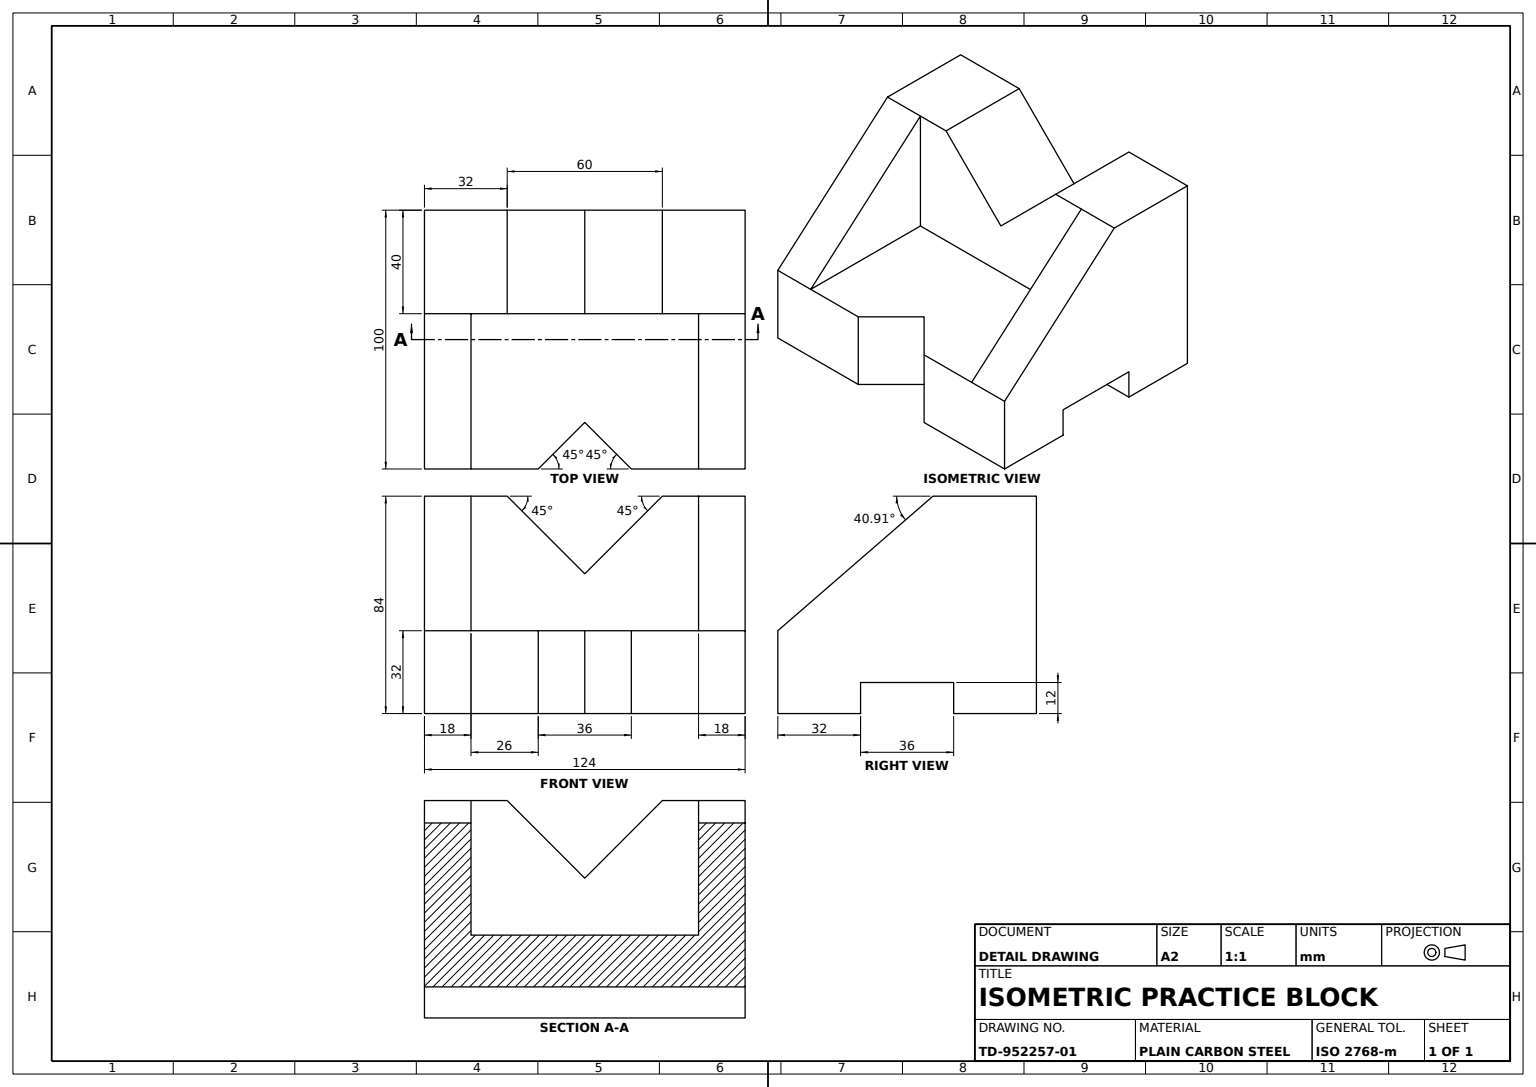
SolidWorks part; units mm, degrees
material "Plain Carbon Steel"
ref_plane "Front Plane" through (0, 0, 0) normal (0, 0, 1) x (1, 0, 0)
ref_plane "Top Plane" through (0, 0, 0) normal (0, 1, 0) x (1, 0, 0)
ref_plane "Right Plane" through (0, 0, 0) normal (1, 0, 0) x (0, 0, -1)
sketch "Block Profile Sketch" plane through (0, 0, 0) normal (0, 0, 1) x (1, 0, 0)
  line L0 (-50, 0) -> (50, 0)
  line L1 (50, 0) -> (50, 32)
  line L2 (50, 32) -> (-10, 84)
  line L3 (-10, 84) -> (-50, 84)
  line L4 (-50, 84) -> (-50, 0)
  dimension "D1" = 100
  dimension "D2" = 50
  dimension "D3" = 40
  dimension "D4" = 32
  dimension "D5" = 84
extrude "Support Block Body" add sketch "Block Profile Sketch" along normal mid plane 124
sketch "Centre Channel Sketch" plane through (0, 0, 0) normal (0, 1, 0) x (1, 0, 0)
  line L0 (-10, -62) -> (-10, 62) construction
  line L1 (-10, 44) -> (50, 44)
  line L2 (-10, 44) -> (-10, -44)
  line L3 (-10, -44) -> (50, -44)
  line L4 (50, 44) -> (50, -44)
  line L5 (50, -62) -> (50, 62) construction
  line L6 (50, 62) -> (-10, 62) construction
  line L7 (50, -62) -> (-10, -62) construction
  dimension "D1" = 18
  dimension "D2" = 18
extrude "Centre Channel Cut" cut sketch "Centre Channel Sketch" along normal blind 124 from offset 32
sketch "V-Notch Sketch" plane through (-10, 0, 0) normal (1, 0, 0) x (0, 0, -1)
  line L0 (30, 84) -> (0, 54)
  line L1 (-44, 84) -> (44, 84) construction
  line L2 (0, 54) -> (-30, 84)
  line L3 (0, 0) -> (0, 54) construction
  line L4 (-62, 0) -> (62, 0) construction
  line L5 (-30, 84) -> (30, 84)
  line L6 (0, 54) -> (0, 84) construction
  dimension "D1" = 30
  dimension "D2" = 60
extrude "V-Notch Cut" cut sketch "V-Notch Sketch" against normal blind 124
sketch "Base Groove Sketch" plane through (0, 32, 0) normal (0, 1, 0) x (1, 0, 0)
  line L0 (50, 18) -> (32, 0)
  line L1 (50, -44) -> (50, 44) construction
  line L2 (32, 0) -> (50, -18)
  line L3 (50, -18) -> (50, 18)
  line L4 (0, 0) -> (50, 0) construction
  dimension "D1" = 18
  dimension "D2" = 36
extrude "Base Groove Cut 18x36" cut sketch "Base Groove Sketch" against normal up to next
sketch "Front Notch Sketch" plane through (0, 0, 62) normal (0, 0, 1) x (1, 0, 0)
  line L0 (-50, 0) -> (50, 0) construction
  line L1 (-18, 0) -> (18, 0)
  line L2 (-18, 0) -> (-18, 12)
  line L3 (-18, 12) -> (18, 12)
  line L4 (18, 0) -> (18, 12)
  line L5 (50, 0) -> (50, 32) construction
  dimension "D1" = 12
  dimension "D2" = 32
  dimension "D3" = 36
extrude "Front Notch Cut" cut sketch "Front Notch Sketch" against normal up to next
